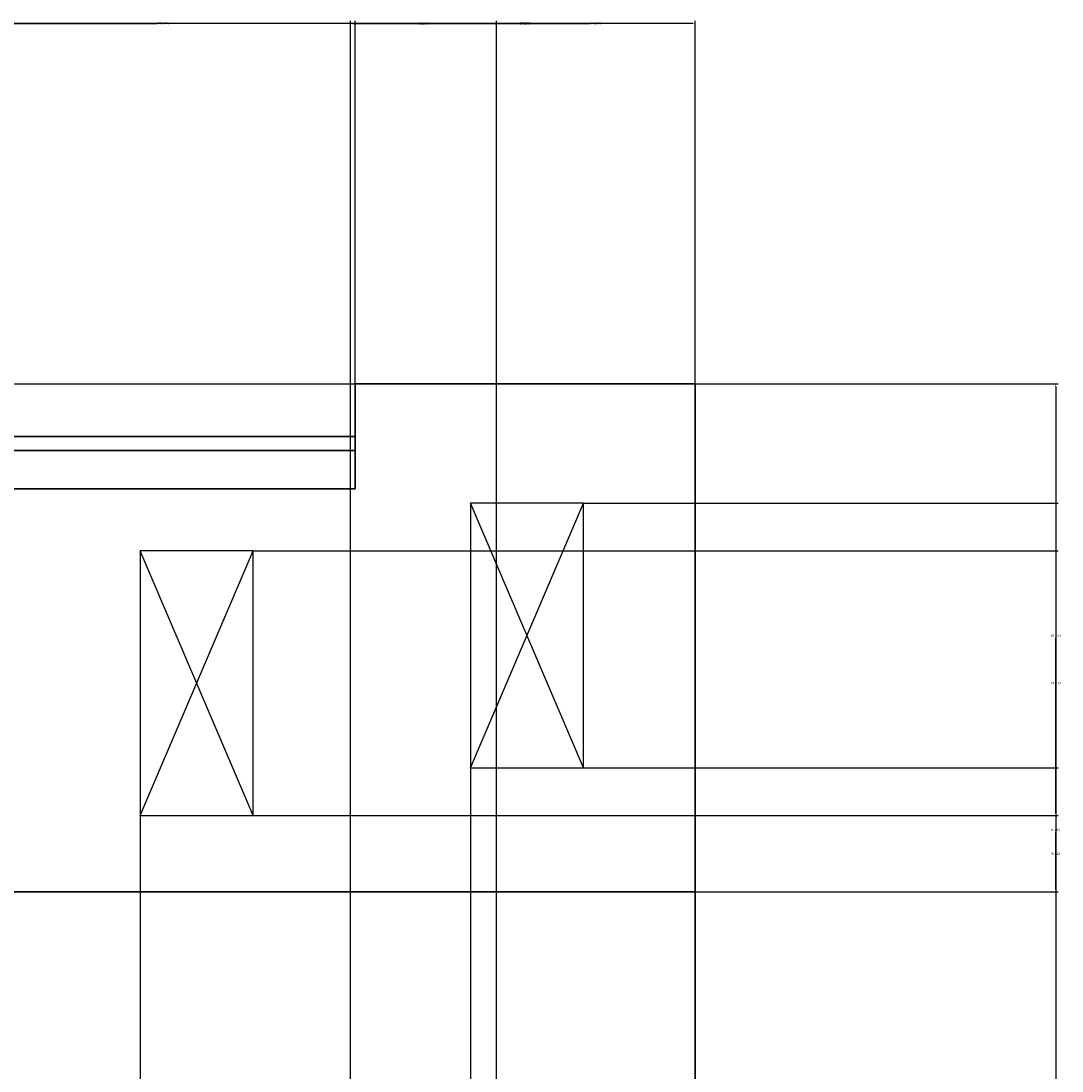
# Model space of a CAD drawing. Units: inches. Extents: x 93 to 565, y 123 to 656.
# Tile 18 of 18: x 491 to 565, y 582 to 656. Entities that reach past the tile are written whole.
import ezdxf

# ---------------------------------------------------------------- set-up
doc = ezdxf.new("R2010")
doc.units = ezdxf.units.IN
doc.header["$MEASUREMENT"] = 0
for name, color, linetype, lineweight in [('A-ANNO-DIMS', 2, 'Continuous', 18), ('A-ELEV', 7, 'Continuous', 35), ('A-GLAZ', 4, 'Continuous', 25)]:
    doc.layers.add(name, color=color, linetype=linetype, lineweight=lineweight)
doc.styles.get("Standard").update_dxf_attribs({"font": 'arial.ttf'})
doc.dimstyles.get("Standard").update_dxf_attribs({"dimtxt": 0.18, "dimasz": 0.18, "dimexe": 0.18, "dimexo": 0.0625, "dimgap": 0.09, "dimtad": 0, "dimtih": 1, "dimtoh": 1, "dimdec": 4, "dimzin": 0, "dimdsep": 46, "dimtxsty": 'Standard', "dimcen": 0.09, "dimadec": 0, "dimazin": 0, "dimtfac": 1, "dimtdec": 4, "dimtofl": 0, "dimtmove": 0, "dimatfit": 3, "dimfxl": 1, "dimtolj": 1, "dimtzin": 0, "dimarcsym": 0})

# ---------------------------------------------------------------- blocks, each defined once
blk = doc.blocks.new('*U9')
for p, q in [((0, 0), (38, 89)), ((38, 0), (0, 89))]:
    blk.add_line(p, q)
blk.add_lwpolyline([(0, 0), (38, 0), (38, 89), (0, 89)], close=True)
blk = doc.blocks.new('*D26')
at = {"layer": 'A-ANNO-DIMS', "color": 0, "lineweight": -2, "transparency": 16777216}
for p, q in [((119.079, 519.162), (119.079, 656.135)), ((119.259, 655.955), (328.787, 655.955)), ((538.899, 655.955), (329.372, 655.955)), ((539.079, 630.467), (539.079, 656.135))]:
    blk.add_line(p, q, dxfattribs=at)
at = {"layer": 'A-ANNO-DIMS', "color": 0, "transparency": 16777216}
for points in [[(119.259, 655.985), (119.259, 655.925), (119.079, 655.955)], [(538.899, 655.985), (538.899, 655.925), (539.079, 655.955)]]:
    blk.add_solid(points, dxfattribs=at)
at = {"layer": 'Defpoints', "color": 0, "transparency": 16777216}
for p in [(539.079, 655.955), (539.079, 630.405), (119.079, 519.1)]:
    blk.add_point(p, dxfattribs=at)
at = {"layer": 'A-ANNO-DIMS', "color": 0, "transparency": 16777216, "insert": (329.079, 655.955), "char_height": 0.18, "attachment_point": 5}
blk.add_mtext('\\A1;420', dxfattribs=at)
blk = doc.blocks.new('*D30')
at = {"layer": 'A-ANNO-DIMS', "color": 0, "lineweight": -2, "transparency": 16777216}
for p, q in [((437.189, 594.342), (437.189, 134.002)), ((539.079, 159.67), (539.079, 134.002)), ((437.369, 134.182), (487.749, 134.182)), ((538.899, 134.182), (488.519, 134.182))]:
    blk.add_line(p, q, dxfattribs=at)
at = {"layer": 'A-ANNO-DIMS', "color": 0, "transparency": 16777216}
for points in [[(437.369, 134.212), (437.369, 134.152), (437.189, 134.182)], [(538.899, 134.212), (538.899, 134.152), (539.079, 134.182)]]:
    blk.add_solid(points, dxfattribs=at)
at = {"layer": 'Defpoints', "color": 0, "transparency": 16777216}
for p in [(437.189, 594.405), (539.079, 159.732), (539.079, 134.182)]:
    blk.add_point(p, dxfattribs=at)
at = {"layer": 'A-ANNO-DIMS', "color": 0, "transparency": 16777216, "insert": (488.134, 134.182), "char_height": 0.18, "attachment_point": 5}
blk.add_mtext('\\A1;101.9', dxfattribs=at)
blk = doc.blocks.new('*D31')
at = {"layer": 'A-ANNO-DIMS', "color": 0, "lineweight": -2, "transparency": 16777216}
for p, q in [((417.872, 630.405), (564.809, 630.405)), ((564.629, 630.225), (564.629, 395.25)), ((564.629, 159.912), (564.629, 394.887)), ((119.142, 159.732), (564.809, 159.732))]:
    blk.add_line(p, q, dxfattribs=at)
at = {"layer": 'A-ANNO-DIMS', "color": 0, "transparency": 16777216}
for points in [[(564.599, 630.225), (564.659, 630.225), (564.629, 630.405)], [(564.599, 159.912), (564.659, 159.912), (564.629, 159.732)]]:
    blk.add_solid(points, dxfattribs=at)
at = {"layer": 'Defpoints', "color": 0, "transparency": 16777216}
for p in [(417.81, 630.405), (564.629, 630.405), (119.079, 159.732)]:
    blk.add_point(p, dxfattribs=at)
at = {"layer": 'A-ANNO-DIMS', "color": 0, "transparency": 16777216, "insert": (564.629, 395.069), "char_height": 0.18, "attachment_point": 5}
blk.add_mtext('\\A1;470.7', dxfattribs=at)
blk = doc.blocks.new('*D88')
at = {"layer": 'A-ANNO-DIMS', "color": 0, "lineweight": -2, "transparency": 16777216}
for p, q in [((487.795, 623.034), (487.795, 656.135)), ((487.975, 655.955), (500.917, 655.955)), ((514.789, 655.955), (501.847, 655.955)), ((514.969, 630.467), (514.969, 656.135))]:
    blk.add_line(p, q, dxfattribs=at)
at = {"layer": 'A-ANNO-DIMS', "color": 0, "transparency": 16777216}
for points in [[(487.975, 655.985), (487.975, 655.925), (487.795, 655.955)], [(514.789, 655.985), (514.789, 655.925), (514.969, 655.955)]]:
    blk.add_solid(points, dxfattribs=at)
at = {"layer": 'Defpoints', "color": 0, "transparency": 16777216}
for p in [(514.969, 655.955), (514.969, 630.405), (487.795, 622.971)]:
    blk.add_point(p, dxfattribs=at)
at = {"layer": 'A-ANNO-DIMS', "color": 0, "transparency": 16777216, "insert": (501.382, 655.955), "char_height": 0.18, "attachment_point": 5}
blk.add_mtext('\\A1;27.174', dxfattribs=at)
blk = doc.blocks.new('*D89')
at = {"layer": 'A-ANNO-DIMS', "color": 0, "lineweight": -2, "transparency": 16777216}
for p, q in [((514.969, 630.467), (514.969, 656.135)), ((515.149, 655.955), (526.646, 655.955)), ((538.899, 655.955), (527.402, 655.955)), ((539.079, 630.467), (539.079, 656.135))]:
    blk.add_line(p, q, dxfattribs=at)
at = {"layer": 'A-ANNO-DIMS', "color": 0, "transparency": 16777216}
for points in [[(515.149, 655.985), (515.149, 655.925), (514.969, 655.955)], [(538.899, 655.985), (538.899, 655.925), (539.079, 655.955)]]:
    blk.add_solid(points, dxfattribs=at)
at = {"layer": 'Defpoints', "color": 0, "transparency": 16777216}
for p in [(539.079, 655.955), (514.969, 630.405), (539.079, 630.405)]:
    blk.add_point(p, dxfattribs=at)
at = {"layer": 'A-ANNO-DIMS', "color": 0, "transparency": 16777216, "insert": (527.024, 655.955), "char_height": 0.18, "attachment_point": 5}
blk.add_mtext('\\A1;24.11', dxfattribs=at)
blk = doc.blocks.new('*D91')
at = {"layer": 'A-ANNO-DIMS', "color": 0, "lineweight": -2, "transparency": 16777216}
for p, q in [((499.729, 599.755), (499.729, 134.002)), ((437.189, 594.342), (437.189, 134.002)), ((437.369, 134.182), (468.065, 134.182)), ((499.549, 134.182), (468.853, 134.182))]:
    blk.add_line(p, q, dxfattribs=at)
at = {"layer": 'A-ANNO-DIMS', "color": 0, "transparency": 16777216}
for points in [[(437.369, 134.212), (437.369, 134.152), (437.189, 134.182)], [(499.549, 134.212), (499.549, 134.152), (499.729, 134.182)]]:
    blk.add_solid(points, dxfattribs=at)
at = {"layer": 'Defpoints', "color": 0, "transparency": 16777216}
for p in [(499.729, 599.817), (437.189, 594.405), (499.729, 134.182)]:
    blk.add_point(p, dxfattribs=at)
at = {"layer": 'A-ANNO-DIMS', "color": 0, "transparency": 16777216, "insert": (468.459, 134.182), "char_height": 0.18, "attachment_point": 5}
blk.add_mtext('\\A1;62.54', dxfattribs=at)
blk = doc.blocks.new('*D92')
at = {"layer": 'A-ANNO-DIMS', "color": 0, "lineweight": -2, "transparency": 16777216}
for p, q in [((523.142, 603.135), (523.142, 134.002)), ((499.729, 599.755), (499.729, 134.002)), ((499.909, 134.182), (510.971, 134.182)), ((522.962, 134.182), (511.9, 134.182))]:
    blk.add_line(p, q, dxfattribs=at)
at = {"layer": 'A-ANNO-DIMS', "color": 0, "transparency": 16777216}
for points in [[(499.909, 134.212), (499.909, 134.152), (499.729, 134.182)], [(522.962, 134.212), (522.962, 134.152), (523.142, 134.182)]]:
    blk.add_solid(points, dxfattribs=at)
at = {"layer": 'Defpoints', "color": 0, "transparency": 16777216}
for p in [(523.142, 603.198), (499.729, 599.817), (523.142, 134.182)]:
    blk.add_point(p, dxfattribs=at)
at = {"layer": 'A-ANNO-DIMS', "color": 0, "transparency": 16777216, "insert": (511.435, 134.182), "char_height": 0.18, "attachment_point": 5}
blk.add_mtext('\\A1;23.412', dxfattribs=at)
blk = doc.blocks.new('*D93')
at = {"layer": 'A-ANNO-DIMS', "color": 0, "lineweight": -2, "transparency": 16777216}
for p, q in [((523.142, 603.135), (523.142, 134.002)), ((539.079, 594.342), (539.079, 134.002)), ((523.322, 134.182), (530.655, 134.182)), ((538.899, 134.182), (531.566, 134.182))]:
    blk.add_line(p, q, dxfattribs=at)
at = {"layer": 'A-ANNO-DIMS', "color": 0, "transparency": 16777216}
for points in [[(523.322, 134.212), (523.322, 134.152), (523.142, 134.182)], [(538.899, 134.212), (538.899, 134.152), (539.079, 134.182)]]:
    blk.add_solid(points, dxfattribs=at)
at = {"layer": 'Defpoints', "color": 0, "transparency": 16777216}
for p in [(523.142, 603.198), (539.079, 594.405), (539.079, 134.182)]:
    blk.add_point(p, dxfattribs=at)
at = {"layer": 'A-ANNO-DIMS', "color": 0, "transparency": 16777216, "insert": (531.11, 134.182), "char_height": 0.18, "attachment_point": 5}
blk.add_mtext('\\A1;15.938', dxfattribs=at)
blk = doc.blocks.new('*D97')
at = {"layer": 'A-ANNO-DIMS', "color": 0, "lineweight": -2, "transparency": 16777216}
for p, q in [((523.204, 603.198), (564.809, 603.198)), ((564.629, 603.018), (564.629, 598.983)), ((564.629, 594.585), (564.629, 598.619)), ((539.142, 594.405), (564.809, 594.405))]:
    blk.add_line(p, q, dxfattribs=at)
at = {"layer": 'A-ANNO-DIMS', "color": 0, "transparency": 16777216}
for points in [[(564.599, 603.018), (564.659, 603.018), (564.629, 603.198)], [(564.599, 594.585), (564.659, 594.585), (564.629, 594.405)]]:
    blk.add_solid(points, dxfattribs=at)
at = {"layer": 'Defpoints', "color": 0, "transparency": 16777216}
for p in [(523.142, 603.198), (564.629, 603.198), (539.079, 594.405)]:
    blk.add_point(p, dxfattribs=at)
at = {"layer": 'A-ANNO-DIMS', "color": 0, "transparency": 16777216, "insert": (564.629, 598.801), "char_height": 0.18, "attachment_point": 5}
blk.add_mtext('\\A1;8.793', dxfattribs=at)
blk = doc.blocks.new('*D98')
at = {"layer": 'A-ANNO-DIMS', "color": 0, "lineweight": -2, "transparency": 16777216}
for p, q in [((531.211, 621.951), (564.809, 621.951)), ((564.629, 621.771), (564.629, 612.757)), ((564.629, 603.378), (564.629, 612.393)), ((523.204, 603.198), (564.809, 603.198))]:
    blk.add_line(p, q, dxfattribs=at)
at = {"layer": 'A-ANNO-DIMS', "color": 0, "transparency": 16777216}
for points in [[(564.599, 621.771), (564.659, 621.771), (564.629, 621.951)], [(564.599, 603.378), (564.659, 603.378), (564.629, 603.198)]]:
    blk.add_solid(points, dxfattribs=at)
at = {"layer": 'Defpoints', "color": 0, "transparency": 16777216}
for p in [(531.149, 621.951), (564.629, 621.951), (523.142, 603.198)]:
    blk.add_point(p, dxfattribs=at)
at = {"layer": 'A-ANNO-DIMS', "color": 0, "transparency": 16777216, "insert": (564.629, 612.575), "char_height": 0.18, "attachment_point": 5}
blk.add_mtext('\\A1;18.753', dxfattribs=at)
blk = doc.blocks.new('*D99')
at = {"layer": 'A-ANNO-DIMS', "color": 0, "lineweight": -2, "transparency": 16777216}
for p, q in [((507.799, 618.571), (564.809, 618.571)), ((564.629, 618.391), (564.629, 609.376)), ((564.629, 599.997), (564.629, 609.012)), ((507.799, 599.817), (564.809, 599.817))]:
    blk.add_line(p, q, dxfattribs=at)
at = {"layer": 'A-ANNO-DIMS', "color": 0, "transparency": 16777216}
for points in [[(564.599, 618.391), (564.659, 618.391), (564.629, 618.571)], [(564.599, 599.997), (564.659, 599.997), (564.629, 599.817)]]:
    blk.add_solid(points, dxfattribs=at)
at = {"layer": 'Defpoints', "color": 0, "transparency": 16777216}
for p in [(507.736, 618.571), (564.629, 618.571), (507.736, 599.817)]:
    blk.add_point(p, dxfattribs=at)
at = {"layer": 'A-ANNO-DIMS', "color": 0, "transparency": 16777216, "insert": (564.629, 609.194), "char_height": 0.18, "attachment_point": 5}
blk.add_mtext('\\A1;18.753', dxfattribs=at)
blk = doc.blocks.new('*D100')
at = {"layer": 'A-ANNO-DIMS', "color": 0, "lineweight": -2, "transparency": 16777216}
for p, q in [((499.792, 599.817), (564.809, 599.817)), ((564.629, 599.637), (564.629, 597.293)), ((564.629, 594.585), (564.629, 596.929)), ((437.251, 594.405), (564.809, 594.405))]:
    blk.add_line(p, q, dxfattribs=at)
at = {"layer": 'A-ANNO-DIMS', "color": 0, "transparency": 16777216}
for points in [[(564.599, 599.637), (564.659, 599.637), (564.629, 599.817)], [(564.599, 594.585), (564.659, 594.585), (564.629, 594.405)]]:
    blk.add_solid(points, dxfattribs=at)
at = {"layer": 'Defpoints', "color": 0, "transparency": 16777216}
for p in [(499.729, 599.817), (437.189, 594.405), (564.629, 594.405)]:
    blk.add_point(p, dxfattribs=at)
at = {"layer": 'A-ANNO-DIMS', "color": 0, "transparency": 16777216, "insert": (564.629, 597.111), "char_height": 0.18, "attachment_point": 5}
blk.add_mtext('\\A1;5.412', dxfattribs=at)
blk = doc.blocks.new('*D105')
at = {"layer": 'A-ANNO-DIMS', "color": 0, "lineweight": -2, "transparency": 16777216}
for p, q in [((119.079, 519.162), (119.079, 656.135)), ((119.259, 655.955), (328.542, 655.955)), ((538.899, 655.955), (329.616, 655.955)), ((539.079, 630.467), (539.079, 656.135))]:
    blk.add_line(p, q, dxfattribs=at)
at = {"layer": 'A-ANNO-DIMS', "color": 0, "transparency": 16777216}
for points in [[(119.259, 655.985), (119.259, 655.925), (119.079, 655.955)], [(538.899, 655.985), (538.899, 655.925), (539.079, 655.955)]]:
    blk.add_solid(points, dxfattribs=at)
at = {"layer": 'Defpoints', "color": 0, "transparency": 16777216}
for p in [(539.079, 655.955), (539.079, 630.405), (119.079, 519.1)]:
    blk.add_point(p, dxfattribs=at)
at = {"layer": 'A-ANNO-DIMS', "color": 0, "transparency": 16777216, "insert": (329.079, 655.955), "char_height": 0.18, "attachment_point": 5}
blk.add_mtext('\\A1;420.000', dxfattribs=at)
blk = doc.blocks.new('*D109')
at = {"layer": 'A-ANNO-DIMS', "color": 0, "lineweight": -2, "transparency": 16777216}
for p, q in [((437.189, 594.342), (437.189, 134.002)), ((539.079, 159.67), (539.079, 134.002)), ((437.369, 134.182), (487.626, 134.182)), ((538.899, 134.182), (488.642, 134.182))]:
    blk.add_line(p, q, dxfattribs=at)
at = {"layer": 'A-ANNO-DIMS', "color": 0, "transparency": 16777216}
for points in [[(437.369, 134.212), (437.369, 134.152), (437.189, 134.182)], [(538.899, 134.212), (538.899, 134.152), (539.079, 134.182)]]:
    blk.add_solid(points, dxfattribs=at)
at = {"layer": 'Defpoints', "color": 0, "transparency": 16777216}
for p in [(437.189, 594.405), (539.079, 159.732), (539.079, 134.182)]:
    blk.add_point(p, dxfattribs=at)
at = {"layer": 'A-ANNO-DIMS', "color": 0, "transparency": 16777216, "insert": (488.134, 134.182), "char_height": 0.18, "attachment_point": 5}
blk.add_mtext('\\A1;101.891', dxfattribs=at)
blk = doc.blocks.new('*D110')
at = {"layer": 'A-ANNO-DIMS', "color": 0, "lineweight": -2, "transparency": 16777216}
for p, q in [((417.872, 630.405), (564.809, 630.405)), ((564.629, 630.225), (564.629, 395.25)), ((564.629, 159.912), (564.629, 394.887)), ((119.142, 159.732), (564.809, 159.732))]:
    blk.add_line(p, q, dxfattribs=at)
at = {"layer": 'A-ANNO-DIMS', "color": 0, "transparency": 16777216}
for points in [[(564.599, 630.225), (564.659, 630.225), (564.629, 630.405)], [(564.599, 159.912), (564.659, 159.912), (564.629, 159.732)]]:
    blk.add_solid(points, dxfattribs=at)
at = {"layer": 'Defpoints', "color": 0, "transparency": 16777216}
for p in [(417.81, 630.405), (564.629, 630.405), (119.079, 159.732)]:
    blk.add_point(p, dxfattribs=at)
at = {"layer": 'A-ANNO-DIMS', "color": 0, "transparency": 16777216, "insert": (564.629, 395.069), "char_height": 0.18, "attachment_point": 5}
blk.add_mtext('\\A1;470.673', dxfattribs=at)
blk = doc.blocks.new('*D167')
at = {"layer": 'A-ANNO-DIMS', "color": 0, "lineweight": -2, "transparency": 16777216}
for p, q in [((487.795, 623.034), (487.795, 656.135)), ((487.975, 655.955), (500.917, 655.955)), ((514.789, 655.955), (501.847, 655.955)), ((514.969, 630.467), (514.969, 656.135))]:
    blk.add_line(p, q, dxfattribs=at)
at = {"layer": 'A-ANNO-DIMS', "color": 0, "transparency": 16777216}
for points in [[(487.975, 655.985), (487.975, 655.925), (487.795, 655.955)], [(514.789, 655.985), (514.789, 655.925), (514.969, 655.955)]]:
    blk.add_solid(points, dxfattribs=at)
at = {"layer": 'Defpoints', "color": 0, "transparency": 16777216}
for p in [(514.969, 655.955), (514.969, 630.405), (487.795, 622.971)]:
    blk.add_point(p, dxfattribs=at)
at = {"layer": 'A-ANNO-DIMS', "color": 0, "transparency": 16777216, "insert": (501.382, 655.955), "char_height": 0.18, "attachment_point": 5}
blk.add_mtext('\\A1;27.174', dxfattribs=at)
blk = doc.blocks.new('*D168')
at = {"layer": 'A-ANNO-DIMS', "color": 0, "lineweight": -2, "transparency": 16777216}
for p, q in [((514.969, 630.467), (514.969, 656.135)), ((515.149, 655.955), (526.576, 655.955)), ((538.899, 655.955), (527.472, 655.955)), ((539.079, 630.467), (539.079, 656.135))]:
    blk.add_line(p, q, dxfattribs=at)
at = {"layer": 'A-ANNO-DIMS', "color": 0, "transparency": 16777216}
for points in [[(515.149, 655.985), (515.149, 655.925), (514.969, 655.955)], [(538.899, 655.985), (538.899, 655.925), (539.079, 655.955)]]:
    blk.add_solid(points, dxfattribs=at)
at = {"layer": 'Defpoints', "color": 0, "transparency": 16777216}
for p in [(539.079, 655.955), (514.969, 630.405), (539.079, 630.405)]:
    blk.add_point(p, dxfattribs=at)
at = {"layer": 'A-ANNO-DIMS', "color": 0, "transparency": 16777216, "insert": (527.024, 655.955), "char_height": 0.18, "attachment_point": 5}
blk.add_mtext('\\A1;24.111', dxfattribs=at)
blk = doc.blocks.new('*D170')
at = {"layer": 'A-ANNO-DIMS', "color": 0, "lineweight": -2, "transparency": 16777216}
for p, q in [((499.729, 599.755), (499.729, 134.002)), ((437.189, 594.342), (437.189, 134.002)), ((437.369, 134.182), (468.012, 134.182)), ((499.549, 134.182), (468.906, 134.182))]:
    blk.add_line(p, q, dxfattribs=at)
at = {"layer": 'A-ANNO-DIMS', "color": 0, "transparency": 16777216}
for points in [[(437.369, 134.212), (437.369, 134.152), (437.189, 134.182)], [(499.549, 134.212), (499.549, 134.152), (499.729, 134.182)]]:
    blk.add_solid(points, dxfattribs=at)
at = {"layer": 'Defpoints', "color": 0, "transparency": 16777216}
for p in [(499.729, 599.817), (437.189, 594.405), (499.729, 134.182)]:
    blk.add_point(p, dxfattribs=at)
at = {"layer": 'A-ANNO-DIMS', "color": 0, "transparency": 16777216, "insert": (468.459, 134.182), "char_height": 0.18, "attachment_point": 5}
blk.add_mtext('\\A1;62.541', dxfattribs=at)
blk = doc.blocks.new('*D171')
at = {"layer": 'A-ANNO-DIMS', "color": 0, "lineweight": -2, "transparency": 16777216}
for p, q in [((523.142, 603.135), (523.142, 134.002)), ((499.729, 599.755), (499.729, 134.002)), ((499.909, 134.182), (510.971, 134.182)), ((522.962, 134.182), (511.9, 134.182))]:
    blk.add_line(p, q, dxfattribs=at)
at = {"layer": 'A-ANNO-DIMS', "color": 0, "transparency": 16777216}
for points in [[(499.909, 134.212), (499.909, 134.152), (499.729, 134.182)], [(522.962, 134.212), (522.962, 134.152), (523.142, 134.182)]]:
    blk.add_solid(points, dxfattribs=at)
at = {"layer": 'Defpoints', "color": 0, "transparency": 16777216}
for p in [(523.142, 603.198), (499.729, 599.817), (523.142, 134.182)]:
    blk.add_point(p, dxfattribs=at)
at = {"layer": 'A-ANNO-DIMS', "color": 0, "transparency": 16777216, "insert": (511.435, 134.182), "char_height": 0.18, "attachment_point": 5}
blk.add_mtext('\\A1;23.412', dxfattribs=at)
blk = doc.blocks.new('*D172')
at = {"layer": 'A-ANNO-DIMS', "color": 0, "lineweight": -2, "transparency": 16777216}
for p, q in [((523.142, 603.135), (523.142, 134.002)), ((539.079, 594.342), (539.079, 134.002)), ((523.322, 134.182), (530.655, 134.182)), ((538.899, 134.182), (531.566, 134.182))]:
    blk.add_line(p, q, dxfattribs=at)
at = {"layer": 'A-ANNO-DIMS', "color": 0, "transparency": 16777216}
for points in [[(523.322, 134.212), (523.322, 134.152), (523.142, 134.182)], [(538.899, 134.212), (538.899, 134.152), (539.079, 134.182)]]:
    blk.add_solid(points, dxfattribs=at)
at = {"layer": 'Defpoints', "color": 0, "transparency": 16777216}
for p in [(523.142, 603.198), (539.079, 594.405), (539.079, 134.182)]:
    blk.add_point(p, dxfattribs=at)
at = {"layer": 'A-ANNO-DIMS', "color": 0, "transparency": 16777216, "insert": (531.11, 134.182), "char_height": 0.18, "attachment_point": 5}
blk.add_mtext('\\A1;15.938', dxfattribs=at)
blk = doc.blocks.new('*D176')
at = {"layer": 'A-ANNO-DIMS', "color": 0, "lineweight": -2, "transparency": 16777216}
for p, q in [((523.204, 603.198), (564.809, 603.198)), ((564.629, 603.018), (564.629, 598.983)), ((564.629, 594.585), (564.629, 598.619)), ((539.142, 594.405), (564.809, 594.405))]:
    blk.add_line(p, q, dxfattribs=at)
at = {"layer": 'A-ANNO-DIMS', "color": 0, "transparency": 16777216}
for points in [[(564.599, 603.018), (564.659, 603.018), (564.629, 603.198)], [(564.599, 594.585), (564.659, 594.585), (564.629, 594.405)]]:
    blk.add_solid(points, dxfattribs=at)
at = {"layer": 'Defpoints', "color": 0, "transparency": 16777216}
for p in [(523.142, 603.198), (564.629, 603.198), (539.079, 594.405)]:
    blk.add_point(p, dxfattribs=at)
at = {"layer": 'A-ANNO-DIMS', "color": 0, "transparency": 16777216, "insert": (564.629, 598.801), "char_height": 0.18, "attachment_point": 5}
blk.add_mtext('\\A1;8.793', dxfattribs=at)
blk = doc.blocks.new('*D177')
at = {"layer": 'A-ANNO-DIMS', "color": 0, "lineweight": -2, "transparency": 16777216}
for p, q in [((531.211, 621.951), (564.809, 621.951)), ((564.629, 621.771), (564.629, 612.757)), ((564.629, 603.378), (564.629, 612.393)), ((523.204, 603.198), (564.809, 603.198))]:
    blk.add_line(p, q, dxfattribs=at)
at = {"layer": 'A-ANNO-DIMS', "color": 0, "transparency": 16777216}
for points in [[(564.599, 621.771), (564.659, 621.771), (564.629, 621.951)], [(564.599, 603.378), (564.659, 603.378), (564.629, 603.198)]]:
    blk.add_solid(points, dxfattribs=at)
at = {"layer": 'Defpoints', "color": 0, "transparency": 16777216}
for p in [(531.149, 621.951), (564.629, 621.951), (523.142, 603.198)]:
    blk.add_point(p, dxfattribs=at)
at = {"layer": 'A-ANNO-DIMS', "color": 0, "transparency": 16777216, "insert": (564.629, 612.575), "char_height": 0.18, "attachment_point": 5}
blk.add_mtext('\\A1;18.753', dxfattribs=at)
blk = doc.blocks.new('*D178')
at = {"layer": 'A-ANNO-DIMS', "color": 0, "lineweight": -2, "transparency": 16777216}
for p, q in [((507.799, 618.571), (564.809, 618.571)), ((564.629, 618.391), (564.629, 609.376)), ((564.629, 599.997), (564.629, 609.012)), ((507.799, 599.817), (564.809, 599.817))]:
    blk.add_line(p, q, dxfattribs=at)
at = {"layer": 'A-ANNO-DIMS', "color": 0, "transparency": 16777216}
for points in [[(564.599, 618.391), (564.659, 618.391), (564.629, 618.571)], [(564.599, 599.997), (564.659, 599.997), (564.629, 599.817)]]:
    blk.add_solid(points, dxfattribs=at)
at = {"layer": 'Defpoints', "color": 0, "transparency": 16777216}
for p in [(507.736, 618.571), (564.629, 618.571), (507.736, 599.817)]:
    blk.add_point(p, dxfattribs=at)
at = {"layer": 'A-ANNO-DIMS', "color": 0, "transparency": 16777216, "insert": (564.629, 609.194), "char_height": 0.18, "attachment_point": 5}
blk.add_mtext('\\A1;18.753', dxfattribs=at)
blk = doc.blocks.new('*D179')
at = {"layer": 'A-ANNO-DIMS', "color": 0, "lineweight": -2, "transparency": 16777216}
for p, q in [((499.792, 599.817), (564.809, 599.817)), ((564.629, 599.637), (564.629, 597.293)), ((564.629, 594.585), (564.629, 596.929)), ((437.251, 594.405), (564.809, 594.405))]:
    blk.add_line(p, q, dxfattribs=at)
at = {"layer": 'A-ANNO-DIMS', "color": 0, "transparency": 16777216}
for points in [[(564.599, 599.637), (564.659, 599.637), (564.629, 599.817)], [(564.599, 594.585), (564.659, 594.585), (564.629, 594.405)]]:
    blk.add_solid(points, dxfattribs=at)
at = {"layer": 'Defpoints', "color": 0, "transparency": 16777216}
for p in [(499.729, 599.817), (437.189, 594.405), (564.629, 594.405)]:
    blk.add_point(p, dxfattribs=at)
at = {"layer": 'A-ANNO-DIMS', "color": 0, "transparency": 16777216, "insert": (564.629, 597.111), "char_height": 0.18, "attachment_point": 5}
blk.add_mtext('\\A1;5.412', dxfattribs=at)
blk = doc.blocks.new('*D185')
at = {"layer": 'A-ANNO-DIMS', "color": 0, "lineweight": -2, "transparency": 16777216}
for p, q in [((514.642, 358.436), (514.642, 656.135)), ((514.822, 655.955), (519.36, 655.955)), ((524.806, 655.955), (520.269, 655.955)), ((524.986, 363.795), (524.986, 656.135))]:
    blk.add_line(p, q, dxfattribs=at)
at = {"layer": 'A-ANNO-DIMS', "color": 0, "transparency": 16777216}
for points in [[(514.822, 655.985), (514.822, 655.925), (514.642, 655.955)], [(524.806, 655.985), (524.806, 655.925), (524.986, 655.955)]]:
    blk.add_solid(points, dxfattribs=at)
at = {"layer": 'Defpoints', "color": 0, "transparency": 16777216}
for p in [(524.986, 655.955), (524.986, 363.732), (514.642, 358.373)]:
    blk.add_point(p, dxfattribs=at)
at = {"layer": 'A-ANNO-DIMS', "color": 0, "transparency": 16777216, "insert": (519.814, 655.955), "char_height": 0.18, "attachment_point": 5}
blk.add_mtext('\\A1;10.344', dxfattribs=at)
blk = doc.blocks.new('*D186')
at = {"layer": 'A-ANNO-DIMS', "color": 0, "lineweight": -2, "transparency": 16777216}
for p, q in [((524.986, 363.795), (524.986, 656.135)), ((525.166, 655.955), (531.578, 655.955)), ((538.899, 655.955), (532.488, 655.955)), ((539.079, 363.795), (539.079, 656.135))]:
    blk.add_line(p, q, dxfattribs=at)
at = {"layer": 'A-ANNO-DIMS', "color": 0, "transparency": 16777216}
for points in [[(525.166, 655.985), (525.166, 655.925), (524.986, 655.955)], [(538.899, 655.985), (538.899, 655.925), (539.079, 655.955)]]:
    blk.add_solid(points, dxfattribs=at)
at = {"layer": 'Defpoints', "color": 0, "transparency": 16777216}
for p in [(539.079, 655.955), (524.986, 363.732), (539.079, 363.732)]:
    blk.add_point(p, dxfattribs=at)
at = {"layer": 'A-ANNO-DIMS', "color": 0, "transparency": 16777216, "insert": (532.033, 655.955), "char_height": 0.18, "attachment_point": 5}
blk.add_mtext('\\A1;14.093', dxfattribs=at)

msp = doc.modelspace()

# ---------------------------------------------------------------- linework, layer by layer
at = {"layer": 'A-ELEV'}
for p, q in [((514.9688, 630.4048), (514.9688, 622.9711)), ((514.9688, 630.4048), (539.0794, 630.4048)), ((539.0794, 630.4048), (539.0794, 594.4048)), ((514.9688, 626.6879), (423.8097, 626.6879)), ((514.9688, 625.6879), (423.8097, 625.6879)), ((514.9688, 622.9711), (487.7953, 622.9711)), ((539.0794, 594.4048), (437.1885, 594.4048)), ((539.0794, 363.7323), (539.0794, 594.4048))]:
    msp.add_line(p, q, dxfattribs=at)

# ---------------------------------------------------------------- block references
at = {"layer": 'A-GLAZ', "xscale": 0.2107133031769033, "yscale": 0.2107133031769033, "zscale": 0.2107133031769033}
for p in [(523.1415, 603.1979), (499.7291, 599.8171)]:
    msp.add_blockref('*U9', p, dxfattribs=at)

# ---------------------------------------------------------------- dimensions: what is measured, and where the dimension line sits
at = {"layer": 'A-ANNO-DIMS'}
for base, p1, p2, override, picture, middle in [((539.0794, 655.9548), (119.0794, 519.0999), (539.0794, 630.4048), {"dimdec": 0, "dimlfac": 1, "dimrnd": 0, "dimzin": 0, "dimdsep": 46, "dimlunit": 2}, '*D26', (329.0794, 655.9548)), ((539.0794, 655.9548), (119.0794, 519.0999), (539.0794, 630.4048), {"dimdec": 3, "dimlfac": 1, "dimrnd": 0, "dimzin": 0, "dimdsep": 46, "dimlunit": 2}, '*D105', (329.0794, 655.9548)), ((514.96884, 655.95478), (487.79526, 622.97108), (514.96884, 630.40477), {"dimdec": 3, "dimlfac": 1, "dimrnd": 0, "dimzin": 0, "dimdsep": 46, "dimlunit": 2}, '*D88', (501.38205, 655.95478)), ((514.96884, 655.95478), (487.79526, 622.97108), (514.96884, 630.40477), {"dimdec": 3, "dimlfac": 1, "dimrnd": 0, "dimzin": 0, "dimdsep": 46, "dimlunit": 2}, '*D167', (501.38205, 655.95478)), ((524.9864, 655.9548), (514.6424, 358.3735), (524.9864, 363.7323), {"dimdec": 3, "dimlfac": 1, "dimrnd": 0, "dimzin": 0, "dimdsep": 46, "dimlunit": 2}, '*D185', (519.8144, 655.9548)), ((539.0794, 655.9548), (514.9688, 630.4048), (539.0794, 630.4048), {"dimdec": 2, "dimlfac": 1, "dimrnd": 0, "dimzin": 0, "dimdsep": 46, "dimlunit": 2}, '*D89', (527.0241, 655.9548)), ((539.0794, 655.9548), (514.9688, 630.4048), (539.0794, 630.4048), {"dimdec": 3, "dimlfac": 1, "dimrnd": 0, "dimzin": 0, "dimdsep": 46, "dimlunit": 2}, '*D168', (527.0241, 655.9548)), ((539.0794, 655.9548), (524.9864, 363.7323), (539.0794, 363.7323), {"dimdec": 3, "dimlfac": 1, "dimrnd": 0, "dimzin": 0, "dimdsep": 46, "dimlunit": 2}, '*D186', (532.0329, 655.9548)), ((523.1415, 134.1823), (499.7291, 599.8171), (523.1415, 603.1979), {"dimdec": 3, "dimlfac": 1, "dimrnd": 0, "dimzin": 0, "dimdsep": 46, "dimlunit": 2}, '*D92', (511.4353, 134.1823)), ((523.1415, 134.1823), (499.7291, 599.8171), (523.1415, 603.1979), {"dimdec": 3, "dimlfac": 1, "dimrnd": 0, "dimzin": 0, "dimdsep": 46, "dimlunit": 2}, '*D171', (511.4353, 134.1823)), ((539.0794, 134.1823), (523.1415, 603.1979), (539.0794, 594.4048), {"dimdec": 3, "dimlfac": 1, "dimrnd": 0, "dimzin": 0, "dimdsep": 46, "dimlunit": 2}, '*D93', (531.1104, 134.1823)), ((539.0794, 134.1823), (523.1415, 603.1979), (539.0794, 594.4048), {"dimdec": 3, "dimlfac": 1, "dimrnd": 0, "dimzin": 0, "dimdsep": 46, "dimlunit": 2}, '*D172', (531.1104, 134.1823)), ((499.7291, 134.1823), (437.1885, 594.4048), (499.7291, 599.8171), {"dimdec": 2, "dimlfac": 1, "dimrnd": 0, "dimzin": 0, "dimdsep": 46, "dimlunit": 2}, '*D91', (468.4588, 134.1823)), ((499.7291, 134.1823), (437.1885, 594.4048), (499.7291, 599.8171), {"dimdec": 3, "dimlfac": 1, "dimrnd": 0, "dimzin": 0, "dimdsep": 46, "dimlunit": 2}, '*D170', (468.4588, 134.1823)), ((539.0794, 134.1823), (437.1885, 594.4048), (539.0794, 159.7323), {"dimdec": 1, "dimlfac": 1, "dimrnd": 0, "dimzin": 0, "dimdsep": 46, "dimlunit": 2}, '*D30', (488.1339, 134.1823)), ((539.0794, 134.1823), (437.1885, 594.4048), (539.0794, 159.7323), {"dimdec": 3, "dimlfac": 1, "dimrnd": 0, "dimzin": 0, "dimdsep": 46, "dimlunit": 2}, '*D109', (488.1339, 134.1823))]:
    dim = msp.add_linear_dim(base=base, p1=p1, p2=p2, dimstyle='Standard', override=override, dxfattribs=at)
    dim.commit()
    dim.dimension.update_dxf_attribs({"geometry": picture, "text_midpoint": middle})
for base, p1, p2, override, picture, middle in [((564.6294, 630.4048), (119.0794, 159.7323), (417.8097, 630.4048), {"dimdec": 1, "dimlfac": 1, "dimrnd": 0, "dimzin": 0, "dimdsep": 46, "dimlunit": 2}, '*D31', (564.6294, 395.0685)), ((564.62936, 630.40478), (119.07936, 159.73225), (417.80971, 630.40477), {"dimdec": 3, "dimlfac": 1, "dimrnd": 0, "dimzin": 0, "dimdsep": 46, "dimlunit": 2}, '*D110', (564.62936, 395.06851)), ((564.62936, 621.95143), (523.14152, 603.19795), (531.14862, 621.95143), {"dimdec": 3, "dimlfac": 1, "dimrnd": 0, "dimzin": 0, "dimdsep": 46, "dimlunit": 2}, '*D98', (564.62936, 612.57469)), ((564.62936, 621.95143), (523.14152, 603.19795), (531.14862, 621.95143), {"dimdec": 3, "dimlfac": 1, "dimrnd": 0, "dimzin": 0, "dimdsep": 46, "dimlunit": 2}, '*D177', (564.62936, 612.57469)), ((564.6294, 618.5705), (507.7362, 599.8171), (507.7362, 618.5705), {"dimdec": 3, "dimlfac": 1, "dimrnd": 0, "dimzin": 0, "dimdsep": 46, "dimlunit": 2}, '*D99', (564.6294, 609.1938)), ((564.6294, 618.5705), (507.7362, 599.8171), (507.7362, 618.5705), {"dimdec": 3, "dimlfac": 1, "dimrnd": 0, "dimzin": 0, "dimdsep": 46, "dimlunit": 2}, '*D178', (564.6294, 609.1938)), ((564.6294, 603.1979), (539.0794, 594.4048), (523.1415, 603.1979), {"dimdec": 3, "dimlfac": 1, "dimrnd": 0, "dimzin": 0, "dimdsep": 46, "dimlunit": 2}, '*D97', (564.6294, 598.8014)), ((564.6294, 603.1979), (539.0794, 594.4048), (523.1415, 603.1979), {"dimdec": 3, "dimlfac": 1, "dimrnd": 0, "dimzin": 0, "dimdsep": 46, "dimlunit": 2}, '*D176', (564.6294, 598.8014)), ((564.6294, 594.4048), (499.7291, 599.8171), (437.1885, 594.4048), {"dimdec": 3, "dimlfac": 1, "dimrnd": 0, "dimzin": 0, "dimdsep": 46, "dimlunit": 2}, '*D100', (564.6294, 597.1109)), ((564.6294, 594.4048), (499.7291, 599.8171), (437.1885, 594.4048), {"dimdec": 3, "dimlfac": 1, "dimrnd": 0, "dimzin": 0, "dimdsep": 46, "dimlunit": 2}, '*D179', (564.6294, 597.1109))]:
    dim = msp.add_linear_dim(base=base, p1=p1, p2=p2, angle=90, dimstyle='Standard', override=override, dxfattribs=at)
    dim.commit()
    dim.dimension.update_dxf_attribs({"geometry": picture, "text_midpoint": middle})

doc.saveas('drawing.dxf')
